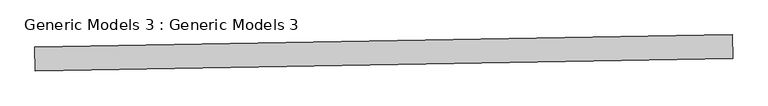
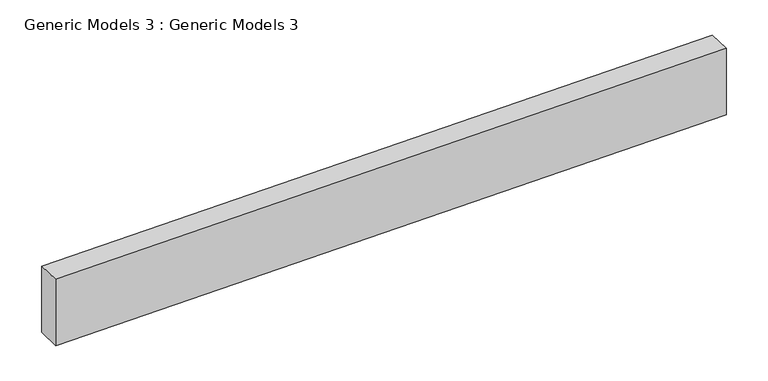
"""IFC4 building model written with IfcOpenShell, lengths in millimetres: proxy geometry, Generic Models 3 : Generic Models 3."""

from ifc_helpers import new_model, si_unit, frame, origin, place, context, project, spatial, polyline, outline, extrude, source, transform, mapped, element, save


def generic_models_3_generic_models_3_fb8d8730(model_context):
    return source(origin(), model_context, "Body", "SweptSolid", [
        extrude(outline(polyline([(8979.3148192, -10872.6535138), (141.4610721, -11026.9188248), (136.1415787, -10722.1652473), (8973.9953257, -10567.8999363), (8979.3148192, -10872.6535138)])), frame((0.0, 0.0, 203.1259248), z_axis=(0.0, 0.0, 1.0), x_axis=(1.0, 0.0, 0.0)), (0.0, 0.0, 1.0), 914.4),
    ])


if __name__ == "__main__":
    model = new_model("IFC4")
    model_context = context("Model", 3, world=origin())
    ifc_project = project(units=[si_unit("LENGTHUNIT", "METRE", prefix="MILLI")], contexts=[model_context])
    site = spatial("IfcSite", under=ifc_project)
    building = spatial("IfcBuilding", under=site)
    placement = place(None, origin())
    generic_models_3_generic_models_3_shape = generic_models_3_generic_models_3_fb8d8730(model_context)
    element("IfcBuildingElementProxy", 1, Name="Generic Models 3 : Generic Models 3", ObjectType="Generic Models 3 : Generic Models 3", at=placement, inside=building, context=model_context, shape_type="MappedRepresentation", body=[
        mapped(generic_models_3_generic_models_3_shape, transform((0.0, 0.0, 0.0), x_axis=(1.0, 0.0, 0.0), y_axis=(0.0, 1.0, 0.0), z_axis=(0.0, 0.0, 1.0))),
    ])
    save(model, "model.ifc")

# Revit data of these elements
# Element 1 (IfcBuildingElementProxy, "Generic Models 3 : Generic Models 3")
#   Materials on its faces: "Parking Stripe"
# Materials
#   "Parking Stripe": class "Paint", colour RGB 250 250 91, transparency 0, Cost = 0
